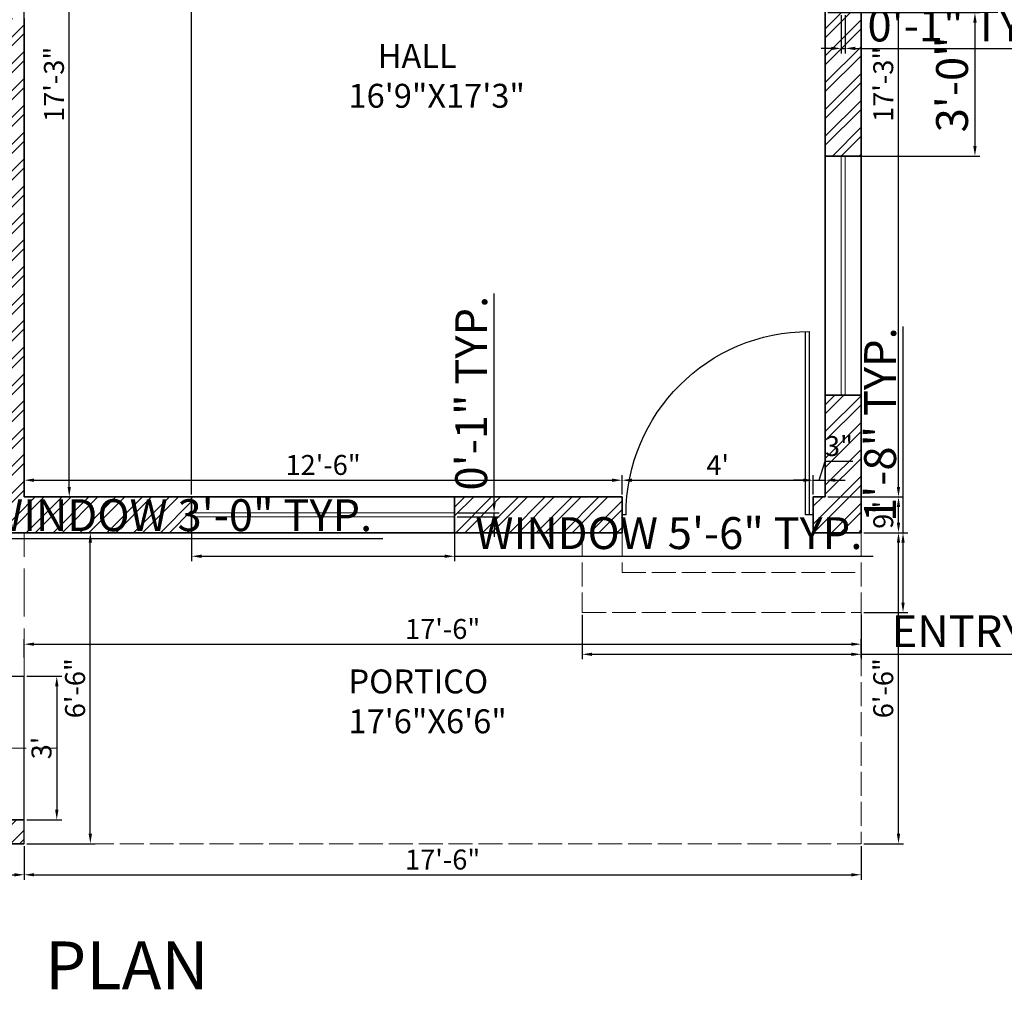
# Model space of a CAD drawing. Units: inches. Extents: x 3595 to 4516, y 2363 to 2965.
# Tile 2 of 12: x 3789 to 4036, y 2363 to 2606. Entities that reach past the tile are written whole.
import ezdxf

# ---------------------------------------------------------------- set-up
doc = ezdxf.new("R2010")
doc.units = ezdxf.units.IN
doc.linetypes.add('ACAD_ISO02W100', pattern=[15, 12, -3])
for name, color, linetype, lineweight in [('A-ANNO-DIMS', 2, 'Continuous', 18), ('A-ANNO-TEXT', 7, 'Continuous', 25), ('A-AREA-IDEN', 7, 'Continuous', 18), ('A-DOOR', 4, 'Continuous', 25), ('A-FLOR-OTLN', 7, 'ACAD_ISO02W100', 18), ('A-FLOR-STRS', 7, 'Continuous', 25), ('A-FLOR-STRS-BYND', 7, 'ACAD_ISO02W100', 18), ('A-FLOR-STRS-OVHD', 7, 'ACAD_ISO02W100', 18), ('A-GLAZ', 4, 'Continuous', 18), ('A-WALL', 7, 'Continuous', 35)]:
    doc.layers.add(name, color=color, linetype=linetype, lineweight=lineweight)
doc.layers.add('A-WALL-PATT', color=251, linetype='Continuous', lineweight=13, true_color=0x636466)
doc.styles.get("Standard").update_dxf_attribs({"font": 'arial.ttf'})
doc.dimstyles.new('ISO-25', dxfattribs={"dimtxt": 8, "dimasz": 2.5, "dimexe": 1.25, "dimexo": 0.625, "dimtad": 1, "dimdec": 1, "dimlunit": 3, "dimtxsty": 'Standard', "dimcen": 2.5, "dimadec": 0, "dimazin": 0, "dimtfac": 1, "dimtdec": 1, "dimtmove": 0, "dimatfit": 3, "dimfxl": 1, "dimarcsym": 0})

# ---------------------------------------------------------------- blocks, each defined once
blk = doc.blocks.new('D')
for p, q in [((1, 0), (1, 46)), ((2, 0), (2, 46)), ((0, 0), (2, 0)), ((47, 0), (48, 0))]:
    blk.add_line(p, q)
at = {"ltscale": 0.5}
blk.add_arc((1, 0), 46, 0, 90, dxfattribs=at)
blk = doc.blocks.new('*D51')
at = {"layer": 'A-ANNO-DIMS', "color": 0, "lineweight": -2, "transparency": 16777216}
for p, q in [((3790.52, 2693.04), (3802.44, 2693.04)), ((3801.19, 2488.54), (3801.19, 2690.54)), ((3790.52, 2486.04), (3802.44, 2486.04))]:
    blk.add_line(p, q, dxfattribs=at)
at = {"layer": 'A-ANNO-DIMS', "color": 0, "transparency": 16777216}
for points in [[(3800.78, 2690.54), (3801.61, 2690.54), (3801.19, 2693.04)], [(3800.78, 2488.54), (3801.61, 2488.54), (3801.19, 2486.04)]]:
    blk.add_solid(points, dxfattribs=at)
at = {"layer": 'Defpoints', "color": 0, "transparency": 16777216}
for p in [(3789.89, 2693.04), (3801.19, 2693.04), (3789.89, 2486.04)]:
    blk.add_point(p, dxfattribs=at)
at = {"layer": 'A-ANNO-DIMS', "color": 0, "transparency": 16777216, "insert": (3798.01, 2589.54), "char_height": 5, "attachment_point": 5, "rotation": 90}
blk.add_mtext('17\'-3"', dxfattribs=at)
blk = doc.blocks.new('*D52')
at = {"layer": 'A-ANNO-DIMS', "color": 0, "lineweight": -2, "transparency": 16777216}
for p, q in [((3789.89, 2486.67), (3789.89, 2491.47)), ((3939.89, 2486.67), (3939.89, 2491.47)), ((3792.39, 2490.22), (3937.39, 2490.22))]:
    blk.add_line(p, q, dxfattribs=at)
at = {"layer": 'A-ANNO-DIMS', "color": 0, "transparency": 16777216}
for points in [[(3792.39, 2490.64), (3792.39, 2489.8), (3789.89, 2490.22)], [(3937.39, 2490.64), (3937.39, 2489.8), (3939.89, 2490.22)]]:
    blk.add_solid(points, dxfattribs=at)
at = {"layer": 'Defpoints', "color": 0, "transparency": 16777216}
for p in [(3939.89, 2490.22), (3789.89, 2486.04), (3939.89, 2486.04)]:
    blk.add_point(p, dxfattribs=at)
at = {"layer": 'A-ANNO-DIMS', "color": 0, "transparency": 16777216, "insert": (3864.89, 2493.4), "char_height": 5, "attachment_point": 5}
blk.add_mtext('12\'-6"', dxfattribs=at)
blk = doc.blocks.new('*D53')
at = {"layer": 'A-ANNO-DIMS', "color": 0, "lineweight": -2, "transparency": 16777216}
for p, q in [((3939.89, 2486.67), (3939.89, 2491.47)), ((3987.89, 2486.67), (3987.89, 2491.47)), ((3942.39, 2490.22), (3985.39, 2490.22))]:
    blk.add_line(p, q, dxfattribs=at)
at = {"layer": 'A-ANNO-DIMS', "color": 0, "transparency": 16777216}
for points in [[(3942.39, 2490.64), (3942.39, 2489.8), (3939.89, 2490.22)], [(3985.39, 2490.64), (3985.39, 2489.8), (3987.89, 2490.22)]]:
    blk.add_solid(points, dxfattribs=at)
at = {"layer": 'Defpoints', "color": 0, "transparency": 16777216}
for p in [(3987.89, 2490.22), (3939.89, 2486.04), (3987.89, 2486.04)]:
    blk.add_point(p, dxfattribs=at)
at = {"layer": 'A-ANNO-DIMS', "color": 0, "transparency": 16777216, "insert": (3963.89, 2493.35), "char_height": 5, "attachment_point": 5}
blk.add_mtext("4'", dxfattribs=at)
blk = doc.blocks.new('*D54')
at = {"layer": 'A-ANNO-DIMS', "color": 0, "lineweight": -2, "transparency": 16777216}
for p, q in [((3989.39, 2490.22), (3990.82, 2494.96)), ((3990.82, 2494.96), (3997.81, 2494.96)), ((3987.89, 2486.67), (3987.89, 2491.47)), ((3990.89, 2486.67), (3990.89, 2491.47)), ((3985.39, 2490.22), (3982.89, 2490.22)), ((3987.89, 2490.22), (3990.89, 2490.22)), ((3987.89, 2490.22), (3990.89, 2490.22)), ((3993.39, 2490.22), (3995.89, 2490.22))]:
    blk.add_line(p, q, dxfattribs=at)
at = {"layer": 'A-ANNO-DIMS', "color": 0, "transparency": 16777216}
for points in [[(3985.39, 2490.64), (3985.39, 2489.8), (3987.89, 2490.22)], [(3993.39, 2490.64), (3993.39, 2489.8), (3990.89, 2490.22)]]:
    blk.add_solid(points, dxfattribs=at)
at = {"layer": 'Defpoints', "color": 0, "transparency": 16777216}
for p in [(3990.89, 2490.22), (3987.89, 2486.04), (3990.89, 2486.04)]:
    blk.add_point(p, dxfattribs=at)
at = {"layer": 'A-ANNO-DIMS', "color": 0, "transparency": 16777216, "insert": (3994.31, 2498.14), "char_height": 5, "attachment_point": 5}
blk.add_mtext('3"', dxfattribs=at)
blk = doc.blocks.new('*D57')
at = {"layer": 'A-ANNO-DIMS', "color": 0, "lineweight": -2, "transparency": 16777216}
for p, q in [((3790.52, 2441.04), (3799.31, 2441.04)), ((3798.06, 2438.54), (3798.06, 2407.54)), ((3790.52, 2405.04), (3799.31, 2405.04))]:
    blk.add_line(p, q, dxfattribs=at)
at = {"layer": 'A-ANNO-DIMS', "color": 0, "transparency": 16777216}
for points in [[(3797.65, 2438.54), (3798.48, 2438.54), (3798.06, 2441.04)], [(3797.65, 2407.54), (3798.48, 2407.54), (3798.06, 2405.04)]]:
    blk.add_solid(points, dxfattribs=at)
at = {"layer": 'Defpoints', "color": 0, "transparency": 16777216}
for p in [(3789.89, 2441.04), (3789.89, 2405.04), (3798.06, 2405.04)]:
    blk.add_point(p, dxfattribs=at)
at = {"layer": 'A-ANNO-DIMS', "color": 0, "transparency": 16777216, "insert": (3794.88, 2423.04), "char_height": 5, "attachment_point": 5, "rotation": 90}
blk.add_mtext("3'", dxfattribs=at)
blk = doc.blocks.new('*D58')
at = {"layer": 'A-ANNO-DIMS', "color": 0, "lineweight": -2, "transparency": 16777216}
for p, q in [((3789.89, 2445.75), (3789.89, 2450.33)), ((3792.39, 2449.08), (3997.39, 2449.08)), ((3999.89, 2445.75), (3999.89, 2450.33))]:
    blk.add_line(p, q, dxfattribs=at)
at = {"layer": 'A-ANNO-DIMS', "color": 0, "transparency": 16777216}
for points in [[(3792.39, 2449.5), (3792.39, 2448.66), (3789.89, 2449.08)], [(3997.39, 2449.5), (3997.39, 2448.66), (3999.89, 2449.08)]]:
    blk.add_solid(points, dxfattribs=at)
at = {"layer": 'Defpoints', "color": 0, "transparency": 16777216}
for p in [(3999.89, 2449.08), (3789.89, 2445.13), (3999.89, 2445.13)]:
    blk.add_point(p, dxfattribs=at)
at = {"layer": 'A-ANNO-DIMS', "color": 0, "transparency": 16777216, "insert": (3894.89, 2452.26), "char_height": 5, "attachment_point": 5}
blk.add_mtext('17\'-6"', dxfattribs=at)
blk = doc.blocks.new('*D59')
at = {"layer": 'A-ANNO-DIMS', "color": 0, "lineweight": -2, "transparency": 16777216}
for p, q in [((3790.52, 2477.04), (3807.73, 2477.04)), ((3806.48, 2401.54), (3806.48, 2474.54)), ((3790.52, 2399.04), (3807.73, 2399.04))]:
    blk.add_line(p, q, dxfattribs=at)
at = {"layer": 'A-ANNO-DIMS', "color": 0, "transparency": 16777216}
for points in [[(3806.06, 2474.54), (3806.9, 2474.54), (3806.48, 2477.04)], [(3806.06, 2401.54), (3806.9, 2401.54), (3806.48, 2399.04)]]:
    blk.add_solid(points, dxfattribs=at)
at = {"layer": 'Defpoints', "color": 0, "transparency": 16777216}
for p in [(3789.89, 2477.04), (3806.48, 2477.04), (3789.89, 2399.04)]:
    blk.add_point(p, dxfattribs=at)
at = {"layer": 'A-ANNO-DIMS', "color": 0, "transparency": 16777216, "insert": (3803.3, 2438.04), "char_height": 5, "attachment_point": 5, "rotation": 90}
blk.add_mtext('6\'-6"', dxfattribs=at)
blk = doc.blocks.new('*D79')
at = {"layer": 'A-ANNO-DIMS', "color": 0, "lineweight": -2, "transparency": 16777216}
for p, q in [((3648.89, 2404.42), (3648.89, 2389.99)), ((3789.89, 2398.42), (3789.89, 2389.99)), ((3651.39, 2391.24), (3787.39, 2391.24))]:
    blk.add_line(p, q, dxfattribs=at)
at = {"layer": 'A-ANNO-DIMS', "color": 0, "transparency": 16777216}
for points in [[(3651.39, 2391.65), (3651.39, 2390.82), (3648.89, 2391.24)], [(3787.39, 2391.65), (3787.39, 2390.82), (3789.89, 2391.24)]]:
    blk.add_solid(points, dxfattribs=at)
at = {"layer": 'Defpoints', "color": 0, "transparency": 16777216}
for p in [(3648.89, 2405.04), (3789.89, 2399.04), (3789.89, 2391.24)]:
    blk.add_point(p, dxfattribs=at)
at = {"layer": 'A-ANNO-DIMS', "color": 0, "transparency": 16777216, "insert": (3719.39, 2394.41), "char_height": 5, "attachment_point": 5}
blk.add_mtext('11\'-9"', dxfattribs=at)
blk = doc.blocks.new('*D80')
at = {"layer": 'A-ANNO-DIMS', "color": 0, "lineweight": -2, "transparency": 16777216}
for p, q in [((3789.89, 2398.42), (3789.89, 2389.99)), ((3999.89, 2398.42), (3999.89, 2389.99)), ((3792.39, 2391.24), (3997.39, 2391.24))]:
    blk.add_line(p, q, dxfattribs=at)
at = {"layer": 'A-ANNO-DIMS', "color": 0, "transparency": 16777216}
for points in [[(3792.39, 2391.65), (3792.39, 2390.82), (3789.89, 2391.24)], [(3997.39, 2391.65), (3997.39, 2390.82), (3999.89, 2391.24)]]:
    blk.add_solid(points, dxfattribs=at)
at = {"layer": 'Defpoints', "color": 0, "transparency": 16777216}
for p in [(3789.89, 2399.04), (3999.89, 2399.04), (3999.89, 2391.24)]:
    blk.add_point(p, dxfattribs=at)
at = {"layer": 'A-ANNO-DIMS', "color": 0, "transparency": 16777216, "insert": (3894.89, 2394.41), "char_height": 5, "attachment_point": 5}
blk.add_mtext('17\'-6"', dxfattribs=at)
blk = doc.blocks.new('*D81')
at = {"layer": 'A-ANNO-DIMS', "color": 0, "lineweight": -2, "transparency": 16777216}
for p, q in [((4000.52, 2477.04), (4010.51, 2477.04)), ((4009.26, 2401.54), (4009.26, 2474.54)), ((4000.52, 2399.04), (4010.51, 2399.04))]:
    blk.add_line(p, q, dxfattribs=at)
at = {"layer": 'A-ANNO-DIMS', "color": 0, "transparency": 16777216}
for points in [[(4008.84, 2474.54), (4009.67, 2474.54), (4009.26, 2477.04)], [(4008.84, 2401.54), (4009.67, 2401.54), (4009.26, 2399.04)]]:
    blk.add_solid(points, dxfattribs=at)
at = {"layer": 'Defpoints', "color": 0, "transparency": 16777216}
for p in [(3999.89, 2477.04), (4009.26, 2477.04), (3999.89, 2399.04)]:
    blk.add_point(p, dxfattribs=at)
at = {"layer": 'A-ANNO-DIMS', "color": 0, "transparency": 16777216, "insert": (4006.08, 2438.04), "char_height": 5, "attachment_point": 5, "rotation": 90}
blk.add_mtext('6\'-6"', dxfattribs=at)
blk = doc.blocks.new('*D82')
at = {"layer": 'A-ANNO-DIMS', "color": 0, "lineweight": -2, "transparency": 16777216}
for p, q in [((3991.52, 2486.04), (4010.51, 2486.04)), ((4009.26, 2479.54), (4009.26, 2483.54)), ((4000.52, 2477.04), (4010.51, 2477.04))]:
    blk.add_line(p, q, dxfattribs=at)
at = {"layer": 'A-ANNO-DIMS', "color": 0, "transparency": 16777216}
for points in [[(4008.84, 2483.54), (4009.67, 2483.54), (4009.26, 2486.04)], [(4008.84, 2479.54), (4009.67, 2479.54), (4009.26, 2477.04)]]:
    blk.add_solid(points, dxfattribs=at)
at = {"layer": 'Defpoints', "color": 0, "transparency": 16777216}
for p in [(3990.89, 2486.04), (4009.26, 2486.04), (3999.89, 2477.04)]:
    blk.add_point(p, dxfattribs=at)
at = {"layer": 'A-ANNO-DIMS', "color": 0, "transparency": 16777216, "insert": (4006.08, 2481.54), "char_height": 5, "attachment_point": 5, "rotation": 90}
blk.add_mtext('9"', dxfattribs=at)
blk = doc.blocks.new('*D83')
at = {"layer": 'A-ANNO-DIMS', "color": 0, "lineweight": -2, "transparency": 16777216}
for p, q in [((3991.52, 2693.04), (4010.51, 2693.04)), ((4009.26, 2488.54), (4009.26, 2690.54)), ((3991.52, 2486.04), (4010.51, 2486.04))]:
    blk.add_line(p, q, dxfattribs=at)
at = {"layer": 'A-ANNO-DIMS', "color": 0, "transparency": 16777216}
for points in [[(4008.84, 2690.54), (4009.67, 2690.54), (4009.26, 2693.04)], [(4008.84, 2488.54), (4009.67, 2488.54), (4009.26, 2486.04)]]:
    blk.add_solid(points, dxfattribs=at)
at = {"layer": 'Defpoints', "color": 0, "transparency": 16777216}
for p in [(3990.89, 2693.04), (4009.26, 2693.04), (3990.89, 2486.04)]:
    blk.add_point(p, dxfattribs=at)
at = {"layer": 'A-ANNO-DIMS', "color": 0, "transparency": 16777216, "insert": (4006.08, 2589.54), "char_height": 5, "attachment_point": 5, "rotation": 90}
blk.add_mtext('17\'-3"', dxfattribs=at)
blk = doc.blocks.new('WIN-GLAZING-66IN')
for p, q in [((0, 1), (66, 1)), ((0, 0), (66, 0))]:
    blk.add_line(p, q)
blk = doc.blocks.new('WIN-GLAZING-60IN')
for p, q in [((0, 60), (0, 0)), ((1, 60), (1, 0))]:
    blk.add_line(p, q)
blk = doc.blocks.new('PORTICO-ENTRY-STEPS')
at = {"ltscale": 0.5}
for p, q in [((0, 20), (0, 0)), ((10, 20), (10, 10)), ((10, 10), (70, 10)), ((0, 0), (70, 0))]:
    blk.add_line(p, q, dxfattribs=at)
blk = doc.blocks.new('*D101')
at = {"layer": 'A-ANNO-DIMS', "color": 0, "lineweight": -2, "transparency": 16777216}
for p, q in [((3738.89, 2480.42), (3738.89, 2474.39)), ((3774.89, 2480.42), (3774.89, 2474.39)), ((3741.39, 2475.64), (3772.39, 2475.64)), ((3774.89, 2475.64), (3879.88, 2475.64))]:
    blk.add_line(p, q, dxfattribs=at)
at = {"layer": 'A-ANNO-DIMS', "color": 0, "transparency": 16777216}
for points in [[(3741.39, 2476.06), (3741.39, 2475.23), (3738.89, 2475.64)], [(3772.39, 2476.06), (3772.39, 2475.23), (3774.89, 2475.64)]]:
    blk.add_solid(points, dxfattribs=at)
at = {"layer": 'Defpoints', "color": 0, "transparency": 16777216}
for p in [(3738.89, 2481.04), (3774.89, 2481.04), (3774.89, 2475.64)]:
    blk.add_point(p, dxfattribs=at)
at = {"layer": 'A-ANNO-DIMS', "color": 0, "transparency": 16777216, "insert": (3828.63, 2480.41), "char_height": 8, "attachment_point": 5}
blk.add_mtext('WINDOW 3\'-0" TYP.', dxfattribs=at)
blk = doc.blocks.new('*D104')
at = {"layer": 'A-ANNO-DIMS', "color": 0, "lineweight": -2, "transparency": 16777216}
for p, q in [((3994.89, 2606.92), (3994.89, 2597.29)), ((3995.89, 2606.92), (3995.89, 2597.29)), ((3992.39, 2598.54), (3989.89, 2598.54)), ((3994.89, 2598.54), (3995.89, 2598.54)), ((3998.39, 2598.54), (4050.91, 2598.54))]:
    blk.add_line(p, q, dxfattribs=at)
at = {"layer": 'A-ANNO-DIMS', "color": 0, "transparency": 16777216}
for points in [[(3992.39, 2598.96), (3992.39, 2598.13), (3994.89, 2598.54)], [(3998.39, 2598.96), (3998.39, 2598.13), (3995.89, 2598.54)]]:
    blk.add_solid(points, dxfattribs=at)
at = {"layer": 'Defpoints', "color": 0, "transparency": 16777216}
for p in [(3994.89, 2607.54), (3995.89, 2607.54), (3995.89, 2598.54)]:
    blk.add_point(p, dxfattribs=at)
at = {"layer": 'A-ANNO-DIMS', "color": 0, "transparency": 16777216, "insert": (4025.9, 2603.25), "char_height": 8, "attachment_point": 5}
blk.add_mtext('0\'-1" TYP.', dxfattribs=at)
blk = doc.blocks.new('*D105')
at = {"layer": 'A-ANNO-DIMS', "color": 0, "lineweight": -2, "transparency": 16777216}
for p, q in [((3831.89, 2480.42), (3831.89, 2469.89)), ((3897.89, 2480.42), (3897.89, 2469.89)), ((3834.39, 2471.14), (3895.39, 2471.14)), ((3897.89, 2471.14), (4002.88, 2471.14))]:
    blk.add_line(p, q, dxfattribs=at)
at = {"layer": 'A-ANNO-DIMS', "color": 0, "transparency": 16777216}
for points in [[(3834.39, 2471.56), (3834.39, 2470.73), (3831.89, 2471.14)], [(3895.39, 2471.56), (3895.39, 2470.73), (3897.89, 2471.14)]]:
    blk.add_solid(points, dxfattribs=at)
at = {"layer": 'Defpoints', "color": 0, "transparency": 16777216}
for p in [(3831.89, 2481.04), (3897.89, 2481.04), (3897.89, 2471.14)]:
    blk.add_point(p, dxfattribs=at)
at = {"layer": 'A-ANNO-DIMS', "color": 0, "transparency": 16777216, "insert": (3951.63, 2475.91), "char_height": 8, "attachment_point": 5}
blk.add_mtext('WINDOW 5\'-6" TYP.', dxfattribs=at)
blk = doc.blocks.new('*D106')
at = {"layer": 'A-ANNO-DIMS', "color": 0, "lineweight": -2, "transparency": 16777216}
for p, q in [((3907.79, 2484.54), (3907.79, 2537.06)), ((3898.52, 2482.04), (3909.04, 2482.04)), ((3898.52, 2481.04), (3909.04, 2481.04)), ((3907.79, 2481.04), (3907.79, 2482.04)), ((3907.79, 2478.54), (3907.79, 2476.04))]:
    blk.add_line(p, q, dxfattribs=at)
at = {"layer": 'A-ANNO-DIMS', "color": 0, "transparency": 16777216}
for points in [[(3907.38, 2484.54), (3908.21, 2484.54), (3907.79, 2482.04)], [(3907.38, 2478.54), (3908.21, 2478.54), (3907.79, 2481.04)]]:
    blk.add_solid(points, dxfattribs=at)
at = {"layer": 'Defpoints', "color": 0, "transparency": 16777216}
for p in [(3897.89, 2482.04), (3897.89, 2481.04), (3907.79, 2482.04)]:
    blk.add_point(p, dxfattribs=at)
at = {"layer": 'A-ANNO-DIMS', "color": 0, "transparency": 16777216, "insert": (3903.08, 2512.05), "char_height": 8, "attachment_point": 5, "rotation": 90}
blk.add_mtext('0\'-1" TYP.', dxfattribs=at)
blk = doc.blocks.new('*D117')
at = {"layer": 'A-ANNO-DIMS', "color": 0, "lineweight": -2, "transparency": 16777216}
for p, q in [((3929.89, 2456.42), (3929.89, 2445.29)), ((3999.89, 2456.42), (3999.89, 2445.29)), ((3932.39, 2446.54), (3997.39, 2446.54)), ((3999.89, 2446.54), (4138.93, 2446.54))]:
    blk.add_line(p, q, dxfattribs=at)
at = {"layer": 'A-ANNO-DIMS', "color": 0, "transparency": 16777216}
for points in [[(3932.39, 2446.96), (3932.39, 2446.13), (3929.89, 2446.54)], [(3997.39, 2446.96), (3997.39, 2446.13), (3999.89, 2446.54)]]:
    blk.add_solid(points, dxfattribs=at)
at = {"layer": 'Defpoints', "color": 0, "transparency": 16777216}
for p in [(3929.89, 2457.04), (3999.89, 2457.04), (3999.89, 2446.54)]:
    blk.add_point(p, dxfattribs=at)
at = {"layer": 'A-ANNO-DIMS', "color": 0, "transparency": 16777216, "insert": (4070.66, 2451.31), "char_height": 8, "attachment_point": 5}
blk.add_mtext('ENTRY STEPS 5\'-10" TYP.', dxfattribs=at)
blk = doc.blocks.new('*D118')
at = {"layer": 'A-ANNO-DIMS', "color": 0, "lineweight": -2, "transparency": 16777216}
for p, q in [((4010.39, 2477.04), (4010.39, 2528.8)), ((4000.52, 2477.04), (4011.64, 2477.04)), ((4010.39, 2459.54), (4010.39, 2474.54)), ((4000.52, 2457.04), (4011.64, 2457.04))]:
    blk.add_line(p, q, dxfattribs=at)
at = {"layer": 'A-ANNO-DIMS', "color": 0, "transparency": 16777216}
for points in [[(4009.98, 2474.54), (4010.81, 2474.54), (4010.39, 2477.04)], [(4009.98, 2459.54), (4010.81, 2459.54), (4010.39, 2457.04)]]:
    blk.add_solid(points, dxfattribs=at)
at = {"layer": 'Defpoints', "color": 0, "transparency": 16777216}
for p in [(3999.89, 2477.04), (4010.39, 2477.04), (3999.89, 2457.04)]:
    blk.add_point(p, dxfattribs=at)
at = {"layer": 'A-ANNO-DIMS', "color": 0, "transparency": 16777216, "insert": (4005.68, 2504.17), "char_height": 8, "attachment_point": 5, "rotation": 90}
blk.add_mtext('1\'-8" TYP.', dxfattribs=at)
blk = doc.blocks.new('*D155')
at = {"layer": 'A-ANNO-DIMS', "color": 0, "lineweight": -2, "transparency": 16777216}
for p, q in [((3991.52, 2607.54), (4029.69, 2607.54)), ((4028.44, 2605.04), (4028.44, 2574.04)), ((3991.52, 2571.54), (4029.69, 2571.54))]:
    blk.add_line(p, q, dxfattribs=at)
at = {"layer": 'A-ANNO-DIMS', "color": 0, "transparency": 16777216}
for points in [[(4028.03, 2605.04), (4028.86, 2605.04), (4028.44, 2607.54)], [(4028.03, 2574.04), (4028.86, 2574.04), (4028.44, 2571.54)]]:
    blk.add_solid(points, dxfattribs=at)
at = {"layer": 'Defpoints', "color": 0, "transparency": 16777216}
for p in [(3990.89, 2607.54), (3990.89, 2571.54), (4028.44, 2571.54)]:
    blk.add_point(p, dxfattribs=at)
at = {"layer": 'A-ANNO-DIMS', "color": 0, "transparency": 16777216, "insert": (4023.73, 2589.54), "char_height": 8, "attachment_point": 5, "rotation": 90}
blk.add_mtext('3\'-0"', dxfattribs=at)
blk = doc.blocks.new('*D157')
at = {"layer": 'A-ANNO-DIMS', "color": 0, "lineweight": -2, "transparency": 16777216}
for p, q in [((3789.89, 2486.67), (3789.89, 2932.84)), ((3831.89, 2486.67), (3831.89, 2932.84)), ((3792.39, 2931.59), (3829.39, 2931.59))]:
    blk.add_line(p, q, dxfattribs=at)
at = {"layer": 'A-ANNO-DIMS', "color": 0, "transparency": 16777216}
for points in [[(3792.39, 2932.01), (3792.39, 2931.18), (3789.89, 2931.59)], [(3829.39, 2932.01), (3829.39, 2931.18), (3831.89, 2931.59)]]:
    blk.add_solid(points, dxfattribs=at)
at = {"layer": 'Defpoints', "color": 0, "transparency": 16777216}
for p in [(3831.89, 2931.59), (3789.89, 2486.04), (3831.89, 2486.04)]:
    blk.add_point(p, dxfattribs=at)
at = {"layer": 'A-ANNO-DIMS', "color": 0, "transparency": 16777216, "insert": (3810.89, 2936.31), "char_height": 8, "attachment_point": 5}
blk.add_mtext('3\'-6"', dxfattribs=at)

msp = doc.modelspace()

# ---------------------------------------------------------------- hatches: boundary and pattern name
at = {"layer": 'A-WALL-PATT'}
h = msp.add_hatch(dxfattribs=at)
h.set_pattern_fill('ANSI32', color=256, scale=0.5)
h.paths.add_polyline_path([(3648.89, 2894.04), (3726.89, 2894.04), (3726.89, 2903.04), (3639.89, 2903.04), (3639.89, 2756.04), (3648.89, 2756.04)])
h.paths.add_polyline_path([(3800.39, 2903.04), (3774.89, 2903.04), (3774.89, 2894.04), (3780.89, 2894.04), (3780.89, 2792.04), (3789.89, 2792.04), (3789.89, 2894.04), (3800.39, 2894.04)])
h.paths.add_polyline_path([(3882.89, 2903.04), (3836.39, 2903.04), (3836.39, 2894.04), (3846.89, 2894.04), (3846.89, 2798.04), (3819.89, 2798.04), (3819.89, 2792.04), (3846.89, 2792.04), (3846.89, 2756.04), (3780.89, 2756.04), (3780.89, 2702.04), (3777.89, 2702.04), (3777.89, 2693.04), (3800.39, 2693.04), (3800.39, 2702.04), (3789.89, 2702.04), (3789.89, 2750.04), (3846.89, 2750.04), (3846.89, 2702.04), (3836.39, 2702.04), (3836.39, 2693.04), (3951.89, 2693.04), (3951.89, 2702.04), (3852.89, 2702.04), (3852.89, 2840.04), (3954.89, 2840.04), (3954.89, 2846.04), (3852.89, 2846.04), (3852.89, 2894.04), (3882.89, 2894.04)])
h.paths.add_polyline_path([(3999.89, 2903.04), (3918.89, 2903.04), (3918.89, 2894.04), (3948.89, 2894.04), (3948.89, 2876.04), (3954.89, 2876.04), (3954.89, 2894.04), (3990.89, 2894.04), (3990.89, 2795.04), (3999.89, 2795.04)])
h.paths.add_polyline_path([(3741.89, 2702.04), (3648.89, 2702.04), (3648.89, 2708.04), (3639.89, 2708.04), (3639.89, 2673.54), (3648.89, 2673.54), (3648.89, 2693.04), (3741.89, 2693.04)])
h.paths.add_polyline_path([(3648.89, 2600.04), (3741.89, 2600.04), (3741.89, 2606.04), (3648.89, 2606.04), (3648.89, 2625.54), (3639.89, 2625.54), (3639.89, 2561.04), (3648.89, 2561.04)])
h.paths.add_polyline_path([(3648.89, 2525.04), (3639.89, 2525.04), (3639.89, 2399.04), (3789.89, 2399.04), (3789.89, 2405.04), (3648.89, 2405.04), (3648.89, 2477.04), (3738.89, 2477.04), (3738.89, 2486.04), (3648.89, 2486.04)])
h.paths.add_polyline_path([(3789.89, 2606.04), (3777.89, 2606.04), (3777.89, 2600.04), (3780.89, 2600.04), (3780.89, 2486.04), (3774.89, 2486.04), (3774.89, 2477.04), (3831.89, 2477.04), (3831.89, 2486.04), (3789.89, 2486.04)])
h.paths.add_polyline_path([(3939.89, 2486.04), (3897.89, 2486.04), (3897.89, 2477.04), (3939.89, 2477.04)])
h.paths.add_polyline_path([(3999.89, 2511.54), (3990.89, 2511.54), (3990.89, 2486.04), (3987.89, 2486.04), (3987.89, 2477.04), (3999.89, 2477.04)])
h.paths.add_polyline_path([(3999.89, 2607.54), (3990.89, 2607.54), (3990.89, 2571.54), (3999.89, 2571.54)])
h.paths.add_polyline_path([(3999.89, 2747.04), (3990.89, 2747.04), (3990.89, 2702.04), (3987.89, 2702.04), (3987.89, 2693.04), (3990.89, 2693.04), (3990.89, 2667.54), (3999.89, 2667.54)])

# ---------------------------------------------------------------- linework, layer by layer
at = {"layer": 'A-FLOR-OTLN', "ltscale": 0.5}
for p, q in [((3999.89, 2477.04), (3999.89, 2399.04)), ((3999.89, 2399.04), (3789.89, 2399.04))]:
    msp.add_line(p, q, dxfattribs=at)
at = {"layer": 'A-FLOR-STRS'}
for p in [(3709.89, 2441.04), (3789.89, 2399.04)]:
    msp.add_line(p, (3789.89, 2441.04), dxfattribs=at)
at = {"layer": 'A-FLOR-STRS-OVHD'}
msp.add_line((3789.89, 2441.04), (3789.89, 2477.04), dxfattribs=at)
at = {"layer": 'A-FLOR-STRS-OVHD', "ltscale": 0.5}
msp.add_lwpolyline([(3780.82, 2459.04), (3679.39, 2459.04), (3679.39, 2423.04), (3798.62, 2423.04)], dxfattribs=at)
at = {"layer": 'A-WALL'}
for p, q in [((3990.89, 2693.04), (3990.89, 2486.04)), ((3789.89, 2486.04), (3789.89, 2606.04)), ((3999.89, 2571.54), (3990.89, 2571.54)), ((3999.89, 2511.54), (3990.89, 2511.54)), ((3789.89, 2486.04), (3939.89, 2486.04)), ((3831.89, 2486.04), (3831.89, 2477.04)), ((3897.89, 2486.04), (3897.89, 2477.04)), ((3939.89, 2486.04), (3939.89, 2477.04)), ((3987.89, 2486.04), (3987.89, 2477.04)), ((3987.89, 2486.04), (3990.89, 2486.04)), ((3648.89, 2477.04), (3939.89, 2477.04)), ((3987.89, 2477.04), (3999.89, 2477.04)), ((3648.89, 2405.04), (3789.89, 2405.04))]:
    msp.add_line(p, q, dxfattribs=at)
msp.add_lwpolyline([(3789.89, 2399.04), (3639.89, 2399.04), (3639.89, 2903.04), (3999.89, 2903.04), (3999.89, 2477.04)], dxfattribs=at)

# ---------------------------------------------------------------- block references
at = {"layer": 'A-DOOR', "xscale": -1}
msp.add_blockref('D', (3987.89, 2481.54), dxfattribs=at)
at = {"layer": 'A-FLOR-STRS-BYND'}
msp.add_blockref('PORTICO-ENTRY-STEPS', (3929.89, 2457.04), dxfattribs=at)
at = {"layer": 'A-GLAZ', "rotation": 180}
msp.add_blockref('WIN-GLAZING-60IN', (3995.89, 2571.54), dxfattribs=at)
at = {"layer": 'A-GLAZ'}
msp.add_blockref('WIN-GLAZING-66IN', (3831.89, 2481.04), dxfattribs=at)

# ---------------------------------------------------------------- texts
at = {"layer": 'A-ANNO-TEXT', "insert": (3795.1, 2374.51), "char_height": 12, "attachment_point": 1}
msp.add_mtext_dynamic_manual_height_columns('{\\fTimes New Roman|b0|i0|c0|p18;PLAN}', width=67.3508, gutter_width=12.5, heights=[0], dxfattribs=at)
at = {"layer": 'A-AREA-IDEN', "char_height": 6, "attachment_point": 1}
for s, insert in [('{\\fTimes New Roman|b0|i0|c0|p18;    HALL\\P16\'9"X17\'3"}', (3871.26, 2599.66)), ('{\\fTimes New Roman|b0|i0|c0|p18;PORTICO\\P17\'6"X6\'6"}', (3871.26, 2442.74))]:
    msp.add_mtext_dynamic_manual_height_columns(s, width=67.3508, gutter_width=12.5, heights=[0], dxfattribs=dict(at, insert=insert))

# ---------------------------------------------------------------- dimensions: what is measured, and where the dimension line sits
at = {"layer": 'A-ANNO-DIMS'}
for base, p1, p2, override, picture, middle in [((3831.89, 2931.59), (3789.89, 2486.04), (3831.89, 2486.04), {"dimdec": 1, "dimlfac": 1, "dimrnd": 0, "dimzin": 1, "dimdsep": 46, "dimlunit": 4, "dimfrac": 2}, '*D157', (3810.89, 2936.31)), ((3990.89, 2490.22), (3987.89, 2486.04), (3990.89, 2486.04), {"dimtxt": 5, "dimclrd": 0, "dimclre": 0, "dimclrt": 0, "dimtmove": 1}, '*D54', (3991.44, 2498.14)), ((3939.89, 2490.22), (3789.89, 2486.04), (3939.89, 2486.04), {"dimtxt": 5, "dimclrd": 0, "dimclre": 0, "dimclrt": 0}, '*D52', (3864.89, 2493.4)), ((3987.89, 2490.22), (3939.89, 2486.04), (3987.89, 2486.04), {"dimtxt": 5, "dimclrd": 0, "dimclre": 0, "dimclrt": 0, "dimtmove": 1}, '*D53', (3963.89, 2493.35)), ((3999.89, 2449.08), (3789.89, 2445.13), (3999.89, 2445.13), {"dimtxt": 5, "dimclrd": 0, "dimclre": 0, "dimclrt": 0}, '*D58', (3894.89, 2452.26)), ((3789.89, 2391.24), (3648.89, 2405.04), (3789.89, 2399.04), {"dimtxt": 5, "dimclrd": 0, "dimclre": 0, "dimclrt": 0, "dimtmove": 1}, '*D79', (3719.39, 2394.41)), ((3999.89, 2391.24), (3789.89, 2399.04), (3999.89, 2399.04), {"dimtxt": 5, "dimclrd": 0, "dimclre": 0, "dimclrt": 0, "dimtmove": 1}, '*D80', (3894.89, 2394.41))]:
    dim = msp.add_linear_dim(base=base, p1=p1, p2=p2, dimstyle='ISO-25', override=override, dxfattribs=at)
    dim.commit()
    dim.dimension.update_dxf_attribs({"geometry": picture, "text_midpoint": middle})
for base, p1, p2, override, picture, middle in [((3801.19, 2693.04), (3789.89, 2486.04), (3789.89, 2693.04), {"dimtxt": 5, "dimclrd": 0, "dimclre": 0, "dimclrt": 0}, '*D51', (3798.01, 2589.54)), ((4009.26, 2693.04), (3990.89, 2486.04), (3990.89, 2693.04), {"dimtxt": 5, "dimclrd": 0, "dimclre": 0, "dimclrt": 0, "dimtmove": 1}, '*D83', (4006.08, 2589.54)), ((4028.44, 2571.54), (3990.89, 2607.54), (3990.89, 2571.54), {"dimdec": 1, "dimlfac": 1, "dimrnd": 0, "dimzin": 1, "dimdsep": 46, "dimlunit": 4, "dimfrac": 2}, '*D155', (4023.73, 2589.54)), ((4009.26, 2486.04), (3999.89, 2477.04), (3990.89, 2486.04), {"dimtxt": 5, "dimclrd": 0, "dimclre": 0, "dimclrt": 0, "dimtmove": 1}, '*D82', (4006.08, 2481.54)), ((3806.48, 2477.04), (3789.89, 2399.04), (3789.89, 2477.04), {"dimtxt": 5, "dimclrd": 0, "dimclre": 0, "dimclrt": 0}, '*D59', (3803.3, 2438.04)), ((4009.26, 2477.04), (3999.89, 2399.04), (3999.89, 2477.04), {"dimtxt": 5, "dimclrd": 0, "dimclre": 0, "dimclrt": 0}, '*D81', (4006.08, 2438.04)), ((3798.06, 2405.04), (3789.89, 2441.04), (3789.89, 2405.04), {"dimtxt": 5, "dimclrd": 0, "dimclre": 0, "dimclrt": 0}, '*D57', (3794.88, 2423.04))]:
    dim = msp.add_linear_dim(base=base, p1=p1, p2=p2, angle=90, dimstyle='ISO-25', override=override, dxfattribs=at)
    dim.commit()
    dim.dimension.update_dxf_attribs({"geometry": picture, "text_midpoint": middle})
for base, p1, p2, text, picture, middle in [((3995.89, 2598.54), (3994.89, 2607.54), (3995.89, 2607.54), '<> TYP.', '*D104', (4025.9, 2603.25)), ((3774.89, 2475.64), (3738.89, 2481.04), (3774.89, 2481.04), 'WINDOW <> TYP.', '*D101', (3828.63, 2480.41)), ((3897.89, 2471.14), (3831.89, 2481.04), (3897.89, 2481.04), 'WINDOW <> TYP.', '*D105', (3951.63, 2475.91)), ((3999.89, 2446.54), (3929.89, 2457.04), (3999.89, 2457.04), 'ENTRY STEPS <> TYP.', '*D117', (4070.66, 2451.31))]:
    dim = msp.add_linear_dim(base=base, p1=p1, p2=p2, text=text, dimstyle='ISO-25', override={"dimdec": 1, "dimlfac": 1, "dimrnd": 0, "dimzin": 1, "dimdsep": 46, "dimlunit": 4, "dimfrac": 2}, dxfattribs=at)
    dim.commit()
    dim.dimension.update_dxf_attribs({"geometry": picture, "text_midpoint": middle})
for base, p1, p2, picture, middle in [((3907.79, 2482.04), (3897.89, 2481.04), (3897.89, 2482.04), '*D106', (3903.08, 2512.05)), ((4010.39, 2477.04), (3999.89, 2457.04), (3999.89, 2477.04), '*D118', (4005.68, 2504.17))]:
    dim = msp.add_linear_dim(base=base, p1=p1, p2=p2, angle=90, text='<> TYP.', dimstyle='ISO-25', override={"dimdec": 1, "dimlfac": 1, "dimrnd": 0, "dimzin": 1, "dimdsep": 46, "dimlunit": 4, "dimfrac": 2}, dxfattribs=at)
    dim.commit()
    dim.dimension.update_dxf_attribs({"geometry": picture, "text_midpoint": middle})

doc.saveas('drawing.dxf')
